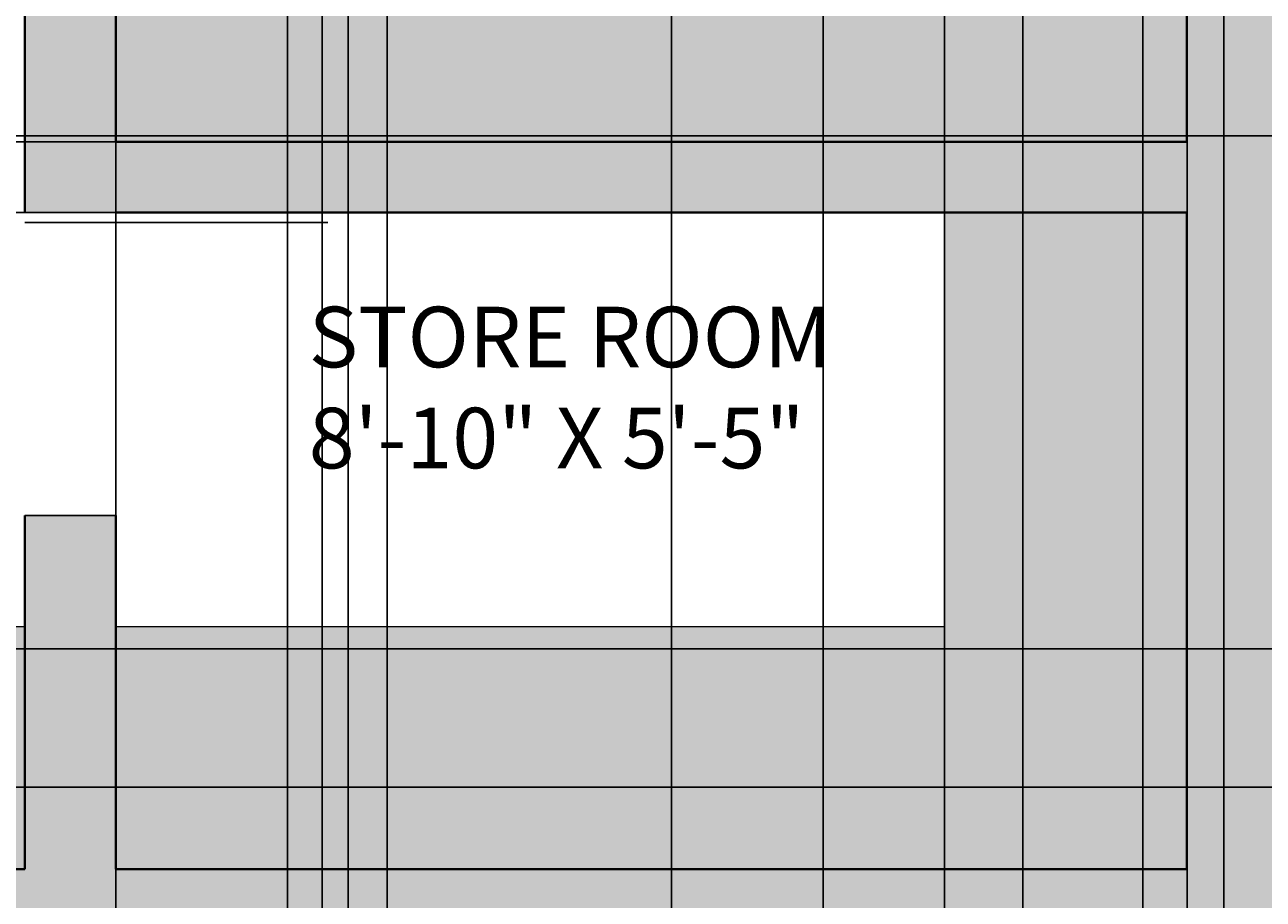
# Model space of a CAD drawing. Units: inches. Extents: x 818 to 1898, y 976 to 2364.
# Tile 88 of 96: x 1591 to 1713, y 1873 to 1960. Entities that reach past the tile are written whole.
import ezdxf

# ---------------------------------------------------------------- set-up
doc = ezdxf.new("R2010")
doc.units = ezdxf.units.IN
doc.header["$LTSCALE"] = 5
doc.header["$MEASUREMENT"] = 0
for name, color, linetype, lineweight in [('A-ANNO-DIMS', 2, 'Continuous', 18), ('A-AREA-IDEN', 7, 'Continuous', 18), ('A-DOOR', 3, 'Continuous', 25), ('A-FLOR-CASE', 8, 'Continuous', 18), ('A-FLOR-CASE-PATT', 33, 'Continuous', 9), ('A-FURN-PATT', 8, 'Continuous', 9), ('A-WALL', 7, 'Continuous', 40)]:
    doc.layers.add(name, color=color, linetype=linetype, lineweight=lineweight)
doc.layers.add('A-WALL-PATT', color=251, linetype='Continuous', lineweight=13, true_color=0x636466)
doc.styles.get("Standard").update_dxf_attribs({"font": 'arial.ttf'})
doc.dimstyles.get("Standard").update_dxf_attribs({"dimtxt": 0.18, "dimasz": 0.18, "dimexe": 0.18, "dimexo": 0.0625, "dimgap": 0.09, "dimtad": 0, "dimtih": 1, "dimtoh": 1, "dimdec": 4, "dimzin": 0, "dimdsep": 46, "dimtxsty": 'Standard', "dimcen": 0.09, "dimadec": 0, "dimazin": 0, "dimtfac": 1, "dimtdec": 4, "dimtofl": 0, "dimtmove": 0, "dimatfit": 3, "dimfxl": 1, "dimtolj": 1, "dimtzin": 0, "dimarcsym": 0})

# ---------------------------------------------------------------- blocks, each defined once
blk = doc.blocks.new('*D85')
at = {"layer": 'A-ANNO-DIMS', "color": 0, "lineweight": -2, "ltscale": 5, "transparency": 16777216}
for p, q in [((1258.79, 2053.08), (1897.92, 2053.08)), ((1897.74, 2052.9), (1897.74, 1876.76)), ((1897.74, 1700.26), (1897.74, 1876.4)), ((1258.79, 1700.08), (1897.92, 1700.08))]:
    blk.add_line(p, q, dxfattribs=at)
at = {"layer": 'A-ANNO-DIMS', "color": 0, "ltscale": 5, "transparency": 16777216}
for points in [[(1897.71, 2052.9), (1897.77, 2052.9), (1897.74, 2053.08)], [(1897.71, 1700.26), (1897.77, 1700.26), (1897.74, 1700.08)]]:
    blk.add_solid(points, dxfattribs=at)
at = {"layer": 'Defpoints', "color": 0, "ltscale": 5, "transparency": 16777216}
for p in [(1258.73, 2053.08), (1897.74, 2053.08), (1258.73, 1700.08)]:
    blk.add_point(p, dxfattribs=at)
at = {"layer": 'A-ANNO-DIMS', "color": 0, "ltscale": 5, "transparency": 16777216, "insert": (1897.74, 1876.58), "char_height": 0.18, "attachment_point": 5}
blk.add_mtext('\\A1;353', dxfattribs=at)
blk = doc.blocks.new('*D102')
at = {"layer": 'A-ANNO-DIMS', "color": 0, "lineweight": -2, "ltscale": 5, "transparency": 16777216}
for p, q in [((1565.48, 1071.12), (1565.48, 2363.87)), ((1565.66, 2363.69), (1595.63, 2363.69)), ((1626.39, 2363.69), (1596.42, 2363.69)), ((1626.57, 1071.12), (1626.57, 2363.87))]:
    blk.add_line(p, q, dxfattribs=at)
at = {"layer": 'A-ANNO-DIMS', "color": 0, "ltscale": 5, "transparency": 16777216}
for points in [[(1565.66, 2363.72), (1565.66, 2363.66), (1565.48, 2363.69)], [(1626.39, 2363.72), (1626.39, 2363.66), (1626.57, 2363.69)]]:
    blk.add_solid(points, dxfattribs=at)
at = {"layer": 'Defpoints', "color": 0, "ltscale": 5, "transparency": 16777216}
for p in [(1626.57, 2363.69), (1565.48, 1071.06), (1626.57, 1071.06)]:
    blk.add_point(p, dxfattribs=at)
at = {"layer": 'A-ANNO-DIMS', "color": 0, "ltscale": 5, "transparency": 16777216, "insert": (1596.03, 2363.69), "char_height": 0.18, "attachment_point": 5}
blk.add_mtext('\\A1;61.09', dxfattribs=at)
blk = doc.blocks.new('*D103')
at = {"layer": 'A-ANNO-DIMS', "color": 0, "lineweight": -2, "ltscale": 5, "transparency": 16777216}
for p, q in [((1626.57, 1071.12), (1626.57, 2363.87)), ((1626.75, 2363.69), (1657.7, 2363.69)), ((1689.29, 2363.69), (1658.35, 2363.69)), ((1689.47, 1071.12), (1689.47, 2363.87))]:
    blk.add_line(p, q, dxfattribs=at)
at = {"layer": 'A-ANNO-DIMS', "color": 0, "ltscale": 5, "transparency": 16777216}
for points in [[(1626.75, 2363.72), (1626.75, 2363.66), (1626.57, 2363.69)], [(1689.29, 2363.72), (1689.29, 2363.66), (1689.47, 2363.69)]]:
    blk.add_solid(points, dxfattribs=at)
at = {"layer": 'Defpoints', "color": 0, "ltscale": 5, "transparency": 16777216}
for p in [(1689.47, 2363.69), (1626.57, 1071.06), (1689.47, 1071.06)]:
    blk.add_point(p, dxfattribs=at)
at = {"layer": 'A-ANNO-DIMS', "color": 0, "ltscale": 5, "transparency": 16777216, "insert": (1658.02, 2363.69), "char_height": 0.18, "attachment_point": 5}
blk.add_mtext('\\A1;62.9', dxfattribs=at)
blk = doc.blocks.new('*D104')
at = {"layer": 'A-ANNO-DIMS', "color": 0, "lineweight": -2, "ltscale": 5, "transparency": 16777216}
for p, q in [((1689.47, 1071.12), (1689.47, 2363.87)), ((1689.65, 2363.69), (1717.4, 2363.69)), ((1745.9, 2363.69), (1718.15, 2363.69)), ((1746.08, 1071.12), (1746.08, 2363.87))]:
    blk.add_line(p, q, dxfattribs=at)
at = {"layer": 'A-ANNO-DIMS', "color": 0, "ltscale": 5, "transparency": 16777216}
for points in [[(1689.65, 2363.72), (1689.65, 2363.66), (1689.47, 2363.69)], [(1745.9, 2363.72), (1745.9, 2363.66), (1746.08, 2363.69)]]:
    blk.add_solid(points, dxfattribs=at)
at = {"layer": 'Defpoints', "color": 0, "ltscale": 5, "transparency": 16777216}
for p in [(1746.08, 2363.69), (1689.47, 1071.06), (1746.08, 1071.06)]:
    blk.add_point(p, dxfattribs=at)
at = {"layer": 'A-ANNO-DIMS', "color": 0, "ltscale": 5, "transparency": 16777216, "insert": (1717.78, 2363.69), "char_height": 0.18, "attachment_point": 5}
blk.add_mtext('\\A1;56.61', dxfattribs=at)
blk = doc.blocks.new('*D121')
at = {"layer": 'A-ANNO-DIMS', "color": 0, "lineweight": -2, "ltscale": 5, "transparency": 16777216}
for p, q in [((1766.29, 1884.2), (818.03, 1884.2)), ((818.21, 1884.02), (818.21, 1841.14)), ((818.21, 1797.9), (818.21, 1840.78)), ((1766.29, 1797.72), (818.03, 1797.72))]:
    blk.add_line(p, q, dxfattribs=at)
at = {"layer": 'A-ANNO-DIMS', "color": 0, "ltscale": 5, "transparency": 16777216}
for points in [[(818.18, 1884.02), (818.24, 1884.02), (818.21, 1884.2)], [(818.18, 1797.9), (818.24, 1797.9), (818.21, 1797.72)]]:
    blk.add_solid(points, dxfattribs=at)
at = {"layer": 'Defpoints', "color": 0, "ltscale": 5, "transparency": 16777216}
for p in [(818.21, 1884.2), (1766.35, 1884.2), (1766.35, 1797.72)]:
    blk.add_point(p, dxfattribs=at)
at = {"layer": 'A-ANNO-DIMS', "color": 0, "ltscale": 5, "transparency": 16777216, "insert": (818.21, 1840.96), "char_height": 0.18, "attachment_point": 5}
blk.add_mtext('\\A1;86.49', dxfattribs=at)
blk = doc.blocks.new('*D154')
at = {"layer": 'A-ANNO-DIMS', "color": 0, "lineweight": -2, "ltscale": 5, "transparency": 16777216}
for p, q in [((1701.37, 1290.14), (1701.37, 2363.87)), ((1701.55, 2363.69), (1705.22, 2363.69)), ((1709.19, 2363.69), (1705.52, 2363.69)), ((1709.37, 1298.14), (1709.37, 2363.87))]:
    blk.add_line(p, q, dxfattribs=at)
at = {"layer": 'A-ANNO-DIMS', "color": 0, "ltscale": 5, "transparency": 16777216}
for points in [[(1701.55, 2363.72), (1701.55, 2363.66), (1701.37, 2363.69)], [(1709.19, 2363.72), (1709.19, 2363.66), (1709.37, 2363.69)]]:
    blk.add_solid(points, dxfattribs=at)
at = {"layer": 'Defpoints', "color": 0, "ltscale": 5, "transparency": 16777216}
for p in [(1709.37, 2363.69), (1709.37, 1298.08), (1701.37, 1290.08)]:
    blk.add_point(p, dxfattribs=at)
at = {"layer": 'A-ANNO-DIMS', "color": 0, "ltscale": 5, "transparency": 16777216, "insert": (1705.37, 2363.69), "char_height": 0.18, "attachment_point": 5}
blk.add_mtext('\\A1;8', dxfattribs=at)
blk = doc.blocks.new('*D173')
at = {"layer": 'A-ANNO-DIMS', "color": 0, "lineweight": -2, "ltscale": 5, "transparency": 16777216}
for p, q in [((1622.73, 1463.14), (1622.73, 2363.87)), ((1622.91, 2363.69), (1638.51, 2363.69)), ((1654.55, 2363.69), (1638.94, 2363.69)), ((1654.73, 1463.14), (1654.73, 2363.87))]:
    blk.add_line(p, q, dxfattribs=at)
at = {"layer": 'A-ANNO-DIMS', "color": 0, "ltscale": 5, "transparency": 16777216}
for points in [[(1622.91, 2363.72), (1622.91, 2363.66), (1622.73, 2363.69)], [(1654.55, 2363.72), (1654.55, 2363.66), (1654.73, 2363.69)]]:
    blk.add_solid(points, dxfattribs=at)
at = {"layer": 'Defpoints', "color": 0, "ltscale": 5, "transparency": 16777216}
for p in [(1654.73, 2363.69), (1622.73, 1463.08), (1654.73, 1463.08)]:
    blk.add_point(p, dxfattribs=at)
at = {"layer": 'A-ANNO-DIMS', "color": 0, "ltscale": 5, "transparency": 16777216, "insert": (1638.73, 2363.69), "char_height": 0.18, "attachment_point": 5}
blk.add_mtext('\\A1;32', dxfattribs=at)
blk = doc.blocks.new('*D174')
at = {"layer": 'A-ANNO-DIMS', "color": 0, "lineweight": -2, "ltscale": 5, "transparency": 16777216}
for p, q in [((1616.73, 1416.75), (1616.73, 2363.87)), ((1616.91, 2363.69), (1619.58, 2363.69)), ((1622.55, 2363.69), (1619.87, 2363.69)), ((1622.73, 1416.75), (1622.73, 2363.87))]:
    blk.add_line(p, q, dxfattribs=at)
at = {"layer": 'A-ANNO-DIMS', "color": 0, "ltscale": 5, "transparency": 16777216}
for points in [[(1616.91, 2363.72), (1616.91, 2363.66), (1616.73, 2363.69)], [(1622.55, 2363.72), (1622.55, 2363.66), (1622.73, 2363.69)]]:
    blk.add_solid(points, dxfattribs=at)
at = {"layer": 'Defpoints', "color": 0, "ltscale": 5, "transparency": 16777216}
for p in [(1622.73, 2363.69), (1616.73, 1416.69), (1622.73, 1416.69)]:
    blk.add_point(p, dxfattribs=at)
at = {"layer": 'A-ANNO-DIMS', "color": 0, "ltscale": 5, "transparency": 16777216, "insert": (1619.73, 2363.69), "char_height": 0.18, "attachment_point": 5}
blk.add_mtext('\\A1;6', dxfattribs=at)
blk = doc.blocks.new('*D175')
at = {"layer": 'A-ANNO-DIMS', "color": 0, "lineweight": -2, "ltscale": 5, "transparency": 16777216}
for p, q in [((1559.73, 1647.64), (1559.73, 2363.87)), ((1559.91, 2363.69), (1614.45, 2363.69)), ((1669.55, 2363.69), (1615.01, 2363.69)), ((1669.73, 1647.64), (1669.73, 2363.87))]:
    blk.add_line(p, q, dxfattribs=at)
at = {"layer": 'A-ANNO-DIMS', "color": 0, "ltscale": 5, "transparency": 16777216}
for points in [[(1559.91, 2363.72), (1559.91, 2363.66), (1559.73, 2363.69)], [(1669.55, 2363.72), (1669.55, 2363.66), (1669.73, 2363.69)]]:
    blk.add_solid(points, dxfattribs=at)
at = {"layer": 'Defpoints', "color": 0, "ltscale": 5, "transparency": 16777216}
for p in [(1669.73, 2363.69), (1559.73, 1647.58), (1669.73, 1647.58)]:
    blk.add_point(p, dxfattribs=at)
at = {"layer": 'A-ANNO-DIMS', "color": 0, "ltscale": 5, "transparency": 16777216, "insert": (1614.73, 2363.69), "char_height": 0.18, "attachment_point": 5}
blk.add_mtext('\\A1;110', dxfattribs=at)
blk = doc.blocks.new('*D195')
at = {"layer": 'A-ANNO-DIMS', "color": 0, "lineweight": -2, "ltscale": 5, "transparency": 16777216}
for p, q in [((1681.73, 1379.14), (1681.73, 2363.87)), ((1681.91, 2363.69), (1693.51, 2363.69)), ((1705.55, 2363.69), (1693.95, 2363.69)), ((1705.73, 1355.14), (1705.73, 2363.87))]:
    blk.add_line(p, q, dxfattribs=at)
at = {"layer": 'A-ANNO-DIMS', "color": 0, "ltscale": 5, "transparency": 16777216}
for points in [[(1681.91, 2363.72), (1681.91, 2363.66), (1681.73, 2363.69)], [(1705.55, 2363.72), (1705.55, 2363.66), (1705.73, 2363.69)]]:
    blk.add_solid(points, dxfattribs=at)
at = {"layer": 'Defpoints', "color": 0, "ltscale": 5, "transparency": 16777216}
for p in [(1705.73, 2363.69), (1681.73, 1379.08), (1705.73, 1355.08)]:
    blk.add_point(p, dxfattribs=at)
at = {"layer": 'A-ANNO-DIMS', "color": 0, "ltscale": 5, "transparency": 16777216, "insert": (1693.73, 2363.69), "char_height": 0.18, "attachment_point": 5}
blk.add_mtext('\\A1;24', dxfattribs=at)
blk = doc.blocks.new('*D203')
at = {"layer": 'A-ANNO-DIMS', "color": 0, "lineweight": -2, "ltscale": 5, "transparency": 16777216}
for p, q in [((1599.73, 1876.14), (1599.73, 2363.87)), ((1599.91, 2363.69), (1652.44, 2363.69)), ((1705.55, 2363.69), (1653.01, 2363.69)), ((1705.73, 1876.14), (1705.73, 2363.87))]:
    blk.add_line(p, q, dxfattribs=at)
at = {"layer": 'A-ANNO-DIMS', "color": 0, "ltscale": 5, "transparency": 16777216}
for points in [[(1599.91, 2363.72), (1599.91, 2363.66), (1599.73, 2363.69)], [(1705.55, 2363.72), (1705.55, 2363.66), (1705.73, 2363.69)]]:
    blk.add_solid(points, dxfattribs=at)
at = {"layer": 'Defpoints', "color": 0, "ltscale": 5, "transparency": 16777216}
for p in [(1705.73, 2363.69), (1599.73, 1876.08), (1705.73, 1876.08)]:
    blk.add_point(p, dxfattribs=at)
at = {"layer": 'A-ANNO-DIMS', "color": 0, "ltscale": 5, "transparency": 16777216, "insert": (1652.73, 2363.69), "char_height": 0.18, "attachment_point": 5}
blk.add_mtext('\\A1;106', dxfattribs=at)
blk = doc.blocks.new('*D204')
at = {"layer": 'A-ANNO-DIMS', "color": 0, "lineweight": -2, "ltscale": 5, "transparency": 16777216}
for p, q in [((1714.79, 2053.08), (1897.92, 2053.08)), ((1897.74, 2052.9), (1897.74, 1960.26)), ((1897.74, 1867.26), (1897.74, 1959.9)), ((1705.79, 1867.08), (1897.92, 1867.08))]:
    blk.add_line(p, q, dxfattribs=at)
at = {"layer": 'A-ANNO-DIMS', "color": 0, "ltscale": 5, "transparency": 16777216}
for points in [[(1897.71, 2052.9), (1897.77, 2052.9), (1897.74, 2053.08)], [(1897.71, 1867.26), (1897.77, 1867.26), (1897.74, 1867.08)]]:
    blk.add_solid(points, dxfattribs=at)
at = {"layer": 'Defpoints', "color": 0, "ltscale": 5, "transparency": 16777216}
for p in [(1714.73, 2053.08), (1897.74, 2053.08), (1705.73, 1867.08)]:
    blk.add_point(p, dxfattribs=at)
at = {"layer": 'A-ANNO-DIMS', "color": 0, "ltscale": 5, "transparency": 16777216, "insert": (1897.74, 1960.08), "char_height": 0.18, "attachment_point": 5}
blk.add_mtext('\\A1;186', dxfattribs=at)
blk = doc.blocks.new('*D211')
at = {"layer": 'A-ANNO-DIMS', "color": 0, "lineweight": -2, "ltscale": 5, "transparency": 16777216}
for p, q in [((1599.66265, 1948.078237), (818.025912, 1948.078237)), ((818.205912, 1947.898237), (818.205912, 1944.758237)), ((818.205912, 1941.258237), (818.205912, 1944.398237)), ((1599.66265, 1941.078237), (818.025912, 1941.078237))]:
    blk.add_line(p, q, dxfattribs=at)
at = {"layer": 'A-ANNO-DIMS', "color": 0, "ltscale": 5, "transparency": 16777216}
for points in [[(818.175912, 1947.898237), (818.235912, 1947.898237), (818.205912, 1948.078237)], [(818.175912, 1941.258237), (818.235912, 1941.258237), (818.205912, 1941.078237)]]:
    blk.add_solid(points, dxfattribs=at)
at = {"layer": 'Defpoints', "color": 0, "ltscale": 5, "transparency": 16777216}
for p in [(818.205912, 1948.078237), (1599.72515, 1948.078237), (1599.72515, 1941.078237)]:
    blk.add_point(p, dxfattribs=at)
at = {"layer": 'A-ANNO-DIMS', "color": 0, "ltscale": 5, "transparency": 16777216, "insert": (818.205912, 1944.578237), "char_height": 0.18, "attachment_point": 5}
blk.add_mtext('\\A1;7', dxfattribs=at)
blk = doc.blocks.new('*D212')
at = {"layer": 'A-ANNO-DIMS', "color": 0, "lineweight": -2, "ltscale": 5, "transparency": 16777216}
for p, q in [((1681.73, 1900.02), (1681.73, 975.66)), ((1705.73, 1876.02), (1705.73, 975.66)), ((1681.91, 975.84), (1693.51, 975.84)), ((1705.55, 975.84), (1693.95, 975.84))]:
    blk.add_line(p, q, dxfattribs=at)
at = {"layer": 'A-ANNO-DIMS', "color": 0, "ltscale": 5, "transparency": 16777216}
for points in [[(1681.91, 975.87), (1681.91, 975.81), (1681.73, 975.84)], [(1705.55, 975.87), (1705.55, 975.81), (1705.73, 975.84)]]:
    blk.add_solid(points, dxfattribs=at)
at = {"layer": 'Defpoints', "color": 0, "ltscale": 5, "transparency": 16777216}
for p in [(1681.73, 1900.08), (1705.73, 1876.08), (1705.73, 975.84)]:
    blk.add_point(p, dxfattribs=at)
at = {"layer": 'A-ANNO-DIMS', "color": 0, "ltscale": 5, "transparency": 16777216, "insert": (1693.73, 975.84), "char_height": 0.18, "attachment_point": 5}
blk.add_mtext('\\A1;24', dxfattribs=at)
blk = doc.blocks.new('*D229')
at = {"layer": 'A-ANNO-DIMS', "color": 0, "lineweight": -2, "ltscale": 5, "transparency": 16777216}
for p, q in [((1599.73, 2044.02), (1599.73, 975.66)), ((1620.14, 2036.06), (1620.14, 975.66)), ((1599.91, 975.84), (1609.47, 975.84)), ((1619.96, 975.84), (1610.4, 975.84))]:
    blk.add_line(p, q, dxfattribs=at)
at = {"layer": 'A-ANNO-DIMS', "color": 0, "ltscale": 5, "transparency": 16777216}
for points in [[(1599.91, 975.87), (1599.91, 975.81), (1599.73, 975.84)], [(1619.96, 975.87), (1619.96, 975.81), (1620.14, 975.84)]]:
    blk.add_solid(points, dxfattribs=at)
at = {"layer": 'Defpoints', "color": 0, "ltscale": 5, "transparency": 16777216}
for p in [(1599.73, 2044.08), (1620.14, 2036.12), (1620.14, 975.84)]:
    blk.add_point(p, dxfattribs=at)
at = {"layer": 'A-ANNO-DIMS', "color": 0, "ltscale": 5, "transparency": 16777216, "insert": (1609.93, 975.84), "char_height": 0.18, "attachment_point": 5}
blk.add_mtext('\\A1;20.416', dxfattribs=at)
blk = doc.blocks.new('*D239')
at = {"layer": 'A-ANNO-DIMS', "color": 0, "lineweight": -2, "ltscale": 5, "transparency": 16777216}
for p, q in [((1483.61, 1979.24), (1897.92, 1979.24)), ((1897.74, 1979.06), (1897.74, 1964.13)), ((1897.74, 1948.84), (1897.74, 1963.77)), ((1483.61, 1948.66), (1897.92, 1948.66))]:
    blk.add_line(p, q, dxfattribs=at)
at = {"layer": 'A-ANNO-DIMS', "color": 0, "ltscale": 5, "transparency": 16777216}
for points in [[(1897.71, 1979.06), (1897.77, 1979.06), (1897.74, 1979.24)], [(1897.71, 1948.84), (1897.77, 1948.84), (1897.74, 1948.66)]]:
    blk.add_solid(points, dxfattribs=at)
at = {"layer": 'Defpoints', "color": 0, "ltscale": 5, "transparency": 16777216}
for p in [(1483.55, 1979.24), (1897.74, 1979.24), (1483.55, 1948.66)]:
    blk.add_point(p, dxfattribs=at)
at = {"layer": 'A-ANNO-DIMS', "color": 0, "ltscale": 5, "transparency": 16777216, "insert": (1897.74, 1963.95), "char_height": 0.18, "attachment_point": 5}
blk.add_mtext('\\A1;30.584', dxfattribs=at)
blk = doc.blocks.new('*D275')
at = {"layer": 'A-ANNO-DIMS', "color": 0, "lineweight": -2, "ltscale": 5, "transparency": 16777216}
for p, q in [((1377.84, 1897.87), (1897.92, 1897.87)), ((1897.74, 1897.69), (1897.74, 1875.99)), ((1897.74, 1853.93), (1897.74, 1875.63)), ((1377.84, 1853.75), (1897.92, 1853.75))]:
    blk.add_line(p, q, dxfattribs=at)
at = {"layer": 'A-ANNO-DIMS', "color": 0, "ltscale": 5, "transparency": 16777216}
for points in [[(1897.71, 1897.69), (1897.77, 1897.69), (1897.74, 1897.87)], [(1897.71, 1853.93), (1897.77, 1853.93), (1897.74, 1853.75)]]:
    blk.add_solid(points, dxfattribs=at)
at = {"layer": 'Defpoints', "color": 0, "ltscale": 5, "transparency": 16777216}
for p in [(1377.78, 1897.87), (1897.74, 1897.87), (1377.78, 1853.75)]:
    blk.add_point(p, dxfattribs=at)
at = {"layer": 'A-ANNO-DIMS', "color": 0, "ltscale": 5, "transparency": 16777216, "insert": (1897.74, 1875.81), "char_height": 0.18, "attachment_point": 5}
blk.add_mtext('\\A1;44.12', dxfattribs=at)
blk = doc.blocks.new('*D282')
at = {"layer": 'A-ANNO-DIMS', "color": 0, "lineweight": -2, "ltscale": 5, "transparency": 16777216}
for p, q in [((1422.08, 2081.19), (1897.92, 2081.19)), ((1897.74, 2081.01), (1897.74, 1884.32)), ((1897.74, 1687.26), (1897.74, 1883.95)), ((1463.79, 1687.08), (1897.92, 1687.08))]:
    blk.add_line(p, q, dxfattribs=at)
at = {"layer": 'A-ANNO-DIMS', "color": 0, "ltscale": 5, "transparency": 16777216}
for points in [[(1897.71, 2081.01), (1897.77, 2081.01), (1897.74, 2081.19)], [(1897.71, 1687.26), (1897.77, 1687.26), (1897.74, 1687.08)]]:
    blk.add_solid(points, dxfattribs=at)
at = {"layer": 'Defpoints', "color": 0, "ltscale": 5, "transparency": 16777216}
for p in [(1422.02, 2081.19), (1897.74, 2081.19), (1463.73, 1687.08)]:
    blk.add_point(p, dxfattribs=at)
at = {"layer": 'A-ANNO-DIMS', "color": 0, "ltscale": 5, "transparency": 16777216, "insert": (1897.74, 1884.13), "char_height": 0.18, "attachment_point": 5}
blk.add_mtext('\\A1;394.1', dxfattribs=at)

msp = doc.modelspace()

# ---------------------------------------------------------------- hatches: boundary and pattern name
at = {"layer": 'A-FLOR-CASE-PATT', "ltscale": 5}
h = msp.add_hatch(color=256, dxfattribs=at)
h.dxf.hatch_style = 1
h.paths.add_polyline_path([(1705.7251, 1941.0782), (1681.7251, 1941.0782), (1681.7251, 1900.0782), (1599.7251, 1900.0782), (1599.7251, 1876.0782), (1705.7251, 1876.0782)])
h.paths.add_polyline_path([(1457.7252, 1409.1177), (1457.7252, 1526.6712), (1439.7252, 1526.6712), (1439.7252, 1457.5313), (1446.3307, 1457.5313), (1446.3307, 1468.9514), (1446.8307, 1470.665), (1446.8307, 1469.665), (1446.8307, 1468.9514), (1446.8307, 1456.8361), (1446.8307, 1444.7258), (1446.8307, 1443.3338), (1446.3307, 1444.7258), (1446.3307, 1456.8361), (1439.7252, 1456.8361), (1439.7252, 1355.0782), (1463.7251, 1355.0782), (1463.7251, 1367.3287), (1458.0475, 1367.3287, -0.23606798), (1457.0475, 1369.3287), (1456.0475, 1369.3287, -0.11764706), (1456.0475, 1386.3287), (1457.0475, 1386.3287, -0.23606798), (1458.0475, 1388.3287), (1463.7251, 1388.3287), (1463.7251, 1389.3211)])
h.paths.add_polyline_path([(1341.2593, 1534.0782), (1246.9377, 1534.0782), (1246.9377, 1510.0782), (1341.2593, 1510.0782)])
h.paths.add_polyline_path([(1288.8272, 1519.927), (1289.8272, 1519.927), (1290.5408, 1519.927), (1302.6561, 1519.927), (1314.7664, 1519.927), (1316.1584, 1519.927), (1314.7664, 1519.427), (1302.6561, 1519.427), (1302.6561, 1512.8214), (1301.9609, 1512.8214), (1301.9609, 1519.427), (1290.5408, 1519.427)], flags=16)
h.paths.add_polyline_path([(1377.7791, 1867.0782), (1344.5531, 1867.0782), (1344.5531, 1860.4726), (1355.9731, 1860.4726), (1357.6867, 1859.9726), (1356.6867, 1859.9726), (1355.9731, 1859.9726), (1343.8579, 1859.9726), (1331.7475, 1859.9726), (1330.3556, 1859.9726), (1331.7475, 1860.4726), (1343.8579, 1860.4726), (1343.8579, 1867.0782), (1311.3271, 1867.0782), (1311.3271, 1853.7496), (1377.7791, 1853.7496)])
h.paths.add_polyline_path([(1301.148, 1610.7299, -0.46196039), (1314.4882, 1599.3725, -0.19222541), (1311.3254, 1591.4497, 0.54791519), (1336.8832, 1607.7707, 0.92061359)])
h.paths.add_polyline_path([(1370.719, 1780.5695, 1), (1332.478, 1780.5695, 1)])
h.paths.add_polyline_path([(1705.7251, 1463.0782), (1681.7251, 1463.0782), (1681.7251, 1379.0782), (1622.7251, 1379.0782), (1622.7251, 1355.0782), (1705.7251, 1355.0782)])
h.paths.add_polyline_path([(1658.1052, 1359.2188), (1658.1786, 1359.2188), (1658.1786, 1373.8763), (1658.1052, 1373.9202)], flags=16)
h.paths.add_polyline_path([(1686.9271, 1409.9311), (1686.8832, 1409.8578), (1701.5845, 1409.8578), (1701.5845, 1409.9311)], flags=16)
h.paths.add_polyline_path([(1637.1266, 1359.2188), (1637.2, 1359.2188), (1637.2, 1373.8763), (1637.1266, 1373.9202)], flags=16)
at = {"layer": 'A-FURN-PATT', "ltscale": 5}
h = msp.add_hatch(color=256, dxfattribs=at)
h.dxf.hatch_style = 1
h.paths.add_polyline_path([(1341.9997, 1981.5338), (1317.9034, 2001.8247), (1314.2595, 2001.8247), (1314.2595, 2004.893), (1310.1046, 2008.3917), (1303.9314, 2008.3917), (1303.9314, 1953.0408), (1308.1629, 1953.0408), (1314.2595, 1958.1746), (1314.2595, 1959.6079), (1315.9616, 1959.6079)])
h.paths.add_polyline_path([(1341.9997, 1981.5338), (1315.9616, 1959.6079), (1336.7936, 1959.6079), (1336.7936, 1953.0408), (1345.3966, 1953.0408), (1345.3966, 1959.6079), (1368.0379, 1959.6079)])
h.paths.add_polyline_path([(1402.518, 2008.3917), (1398.8475, 2008.3917), (1398.8475, 2001.8247), (1376.3134, 2001.8247), (1376.3134, 2008.3917), (1373.8948, 2008.3917), (1367.9307, 2003.3695), (1367.9307, 2001.8247), (1366.0961, 2001.8247), (1341.9997, 1981.5338), (1368.0379, 1959.6079), (1375.8366, 1953.0408), (1376.3134, 1953.0408), (1376.3134, 1959.6079), (1398.8475, 1959.6079), (1398.8475, 1953.0408), (1402.518, 1953.0408)])
h.paths.add_polyline_path([(1366.0961, 2001.8247), (1345.3966, 2001.8247), (1345.3966, 2008.3917), (1336.7936, 2008.3917), (1336.7936, 2001.8247), (1317.9034, 2001.8247), (1341.9997, 1981.5338)])
h.paths.add_polyline_path([(1336.7936, 1959.6079), (1315.9616, 1959.6079), (1314.2595, 1958.1746), (1314.2595, 1953.0408), (1336.7936, 1953.0408)], flags=17)
h.paths.add_polyline_path([(1367.9307, 1959.6079), (1345.3966, 1959.6079), (1345.3966, 1953.0408), (1367.9307, 1953.0408)], flags=17)
h.paths.add_polyline_path([(1398.8475, 1959.6079), (1376.3134, 1959.6079), (1376.3134, 1953.0408), (1398.8475, 1953.0408)], flags=17)
h.paths.add_polyline_path([(1368.0379, 1959.6079), (1367.9307, 1959.6079), (1367.9307, 1953.0408), (1375.8366, 1953.0408)], flags=17)
h.paths.add_polyline_path([(1314.2595, 1958.1746), (1308.1629, 1953.0408), (1314.2595, 1953.0408)], flags=17)
h.paths.add_polyline_path([(1315.9616, 1959.6079), (1314.2595, 1959.6079), (1314.2595, 1958.1746)], flags=16)
h.paths.add_polyline_path([(1314.2595, 2008.3917), (1310.1046, 2008.3917), (1314.2595, 2004.893)], flags=17)
h.paths.add_polyline_path([(1336.7936, 2008.3917), (1314.2595, 2008.3917), (1314.2595, 2004.893), (1317.9034, 2001.8247), (1336.7936, 2001.8247)], flags=17)
h.paths.add_polyline_path([(1314.2595, 2004.893), (1314.2595, 2001.8247), (1317.9034, 2001.8247)], flags=16)
h.paths.add_polyline_path([(1367.9307, 2008.3917), (1345.3966, 2008.3917), (1345.3966, 2001.8247), (1366.0961, 2001.8247), (1367.9307, 2003.3695)], flags=17)
h.paths.add_polyline_path([(1398.8475, 2008.3917), (1376.3134, 2008.3917), (1376.3134, 2001.8247), (1398.8475, 2001.8247)], flags=17)
h.paths.add_polyline_path([(1373.8948, 2008.3917), (1367.9307, 2008.3917), (1367.9307, 2003.3695)], flags=17)
h.paths.add_polyline_path([(1367.9307, 2003.3695), (1366.0961, 2001.8247), (1367.9307, 2001.8247)], flags=16)
h.paths.add_polyline_path([(1546.1595, 2044.0782), (1451.7698, 2044.0782), (1451.7698, 2020.0782), (1546.1595, 2020.0782)])
h.paths.add_polyline_path([(1492.0729, 2040.001, 0.431429), (1491.8238, 2040.251), (1491.3087, 2040.251, 0.41521699), (1491.0729, 2040.001)], flags=16)
h.paths.add_polyline_path([(1481.8346, 2039.6036), (1511.886, 2039.6036), (1511.886, 2024.9917), (1481.8346, 2024.9917)], flags=16)
h.paths.add_polyline_path([(1491.0729, 2039.4857), (1491.0729, 2039.501), (1492.0729, 2039.501, -0.41174844), (1491.8401, 2039.251), (1491.8229, 2039.251), (1491.8229, 2039.2509, 0.43259178), (1492.0729, 2039.501), (1491.0729, 2039.501, 0.43260402), (1491.3229, 2039.2509), (1491.3229, 2039.251), (1491.325, 2039.251, -0.41658228)], flags=0)
h.paths.add_polyline_path([(1485.3701, 2030.9622), (1485.3701, 2034.3556, -0.41421356), (1488.3701, 2037.3556), (1490.3421, 2037.3556, -0.07791932), (1491.0729, 2038.751), (1495.0729, 2038.751, -0.31486788), (1496.07, 2037.1201, -0.30166092), (1497.9049, 2034.3556), (1497.9049, 2030.9622, -0.41421356), (1494.9049, 2027.9622), (1488.3701, 2027.9622, -0.41421356)], flags=0)
h.paths.add_polyline_path([(1490.3229, 2035.751, 0.26556482), (1491.3229, 2036.751), (1491.3229, 2037.126), (1491.0729, 2037.126, -0.79141832), (1490.5434, 2037.251, -0.79141832), (1491.0729, 2037.376), (1491.3229, 2037.376), (1491.3229, 2037.751), (1492.0729, 2037.751), (1492.0729, 2037.376), (1492.3229, 2037.376, -0.79141832), (1492.8524, 2037.251, -0.79141832), (1492.3229, 2037.126), (1492.1491, 2037.126, -0.08662632), (1492.5376, 2036.0294, 0.10704809), (1493.0729, 2035.751), (1490.3229, 2035.751)], flags=0)
h.paths.add_polyline_path([(1491.9774, 2037.251, -1), (1491.4184, 2037.251, -1)], flags=0)
h.paths.add_polyline_path([(1500.0743, 2028.6045), (1500.0743, 2029.4074), (1510.8414, 2029.4074), (1510.8414, 2028.6045)], flags=0)
h.paths.add_polyline_path([(1500.0743, 2030.5314), (1500.0743, 2031.3342), (1510.8414, 2031.3342), (1510.8414, 2030.5314)], flags=0)
h.paths.add_polyline_path([(1500.0743, 2032.94), (1500.0743, 2033.7428), (1510.8414, 2033.7428), (1510.8414, 2032.94)], flags=0)
h.paths.add_polyline_path([(1500.0743, 2035.7499), (1500.0743, 2036.5528), (1510.8414, 2036.5528), (1510.8414, 2035.7499)], flags=0)
h.paths.add_polyline_path([(1590.7252, 2044.0782), (1576.1595, 2044.0782), (1576.1595, 2020.0782), (1590.7252, 2020.0782)])
h.paths.add_polyline_path([(1668.4429, 2044.0782), (1599.7251, 2044.0782), (1599.7251, 2020.0782), (1668.4429, 2020.0782)])
h.paths.add_polyline_path([(1621.2588, 2040.001, 0.431429), (1621.0097, 2040.251), (1620.4946, 2040.251, 0.41521699), (1620.2588, 2040.001)], flags=16)
h.paths.add_polyline_path([(1611.0205, 2024.9917), (1611.0205, 2039.6036), (1641.0719, 2039.6036), (1641.0719, 2024.9917)], flags=16)
h.paths.add_polyline_path([(1620.2588, 2039.4857), (1620.2588, 2039.501), (1621.2588, 2039.501, -0.41174844), (1621.026, 2039.251), (1621.0088, 2039.251), (1621.0088, 2039.2509, 0.43259178), (1621.2588, 2039.501), (1620.2588, 2039.501, 0.43260402), (1620.5088, 2039.2509), (1620.5088, 2039.251), (1620.5109, 2039.251, -0.41658228)], flags=0)
h.paths.add_polyline_path([(1614.556, 2030.9622), (1614.556, 2034.3556, -0.41421356), (1617.556, 2037.3556), (1619.528, 2037.3556, -0.07791932), (1620.2588, 2038.751), (1624.2588, 2038.751, -0.31486788), (1625.2559, 2037.1201, -0.30166092), (1627.0908, 2034.3556), (1627.0908, 2030.9622, -0.41421356), (1624.0908, 2027.9622), (1617.556, 2027.9622, -0.41421356)], flags=0)
h.paths.add_polyline_path([(1619.5088, 2035.751, 0.26556482), (1620.5088, 2036.751), (1620.5088, 2037.126), (1620.2588, 2037.126, -0.79141832), (1619.7293, 2037.251, -0.79141832), (1620.2588, 2037.376), (1620.5088, 2037.376), (1620.5088, 2037.751), (1621.2588, 2037.751), (1621.2588, 2037.376), (1621.5088, 2037.376, -0.79141832), (1622.0383, 2037.251, -0.79141832), (1621.5088, 2037.126), (1621.335, 2037.126, -0.08662632), (1621.7235, 2036.0294, 0.10704809), (1622.2588, 2035.751), (1619.5088, 2035.751)], flags=0)
h.paths.add_polyline_path([(1620.6043, 2037.251, -1), (1621.1633, 2037.251, -1)], flags=0)
h.paths.add_polyline_path([(1629.2602, 2028.6045), (1629.2602, 2029.4074), (1640.0273, 2029.4074), (1640.0273, 2028.6045)], flags=0)
h.paths.add_polyline_path([(1629.2602, 2030.5314), (1629.2602, 2031.3342), (1640.0273, 2031.3342), (1640.0273, 2030.5314)], flags=0)
h.paths.add_polyline_path([(1629.2602, 2032.94), (1629.2602, 2033.7428), (1640.0273, 2033.7428), (1640.0273, 2032.94)], flags=0)
h.paths.add_polyline_path([(1629.2602, 2035.7499), (1629.2602, 2036.5528), (1640.0273, 2036.5528), (1640.0273, 2035.7499)], flags=0)
h.paths.add_polyline_path([(1705.7251, 2044.0782), (1698.4429, 2044.0782), (1698.4429, 2020.0782), (1705.7251, 2020.0782)])
h.paths.add_polyline_path([(1705.7251, 1972.0782), (1599.7251, 1972.0782), (1599.7251, 1948.0782), (1705.7251, 1948.0782)])
h.paths.add_polyline_path([(1550.0109, 1979.2444), (1483.5451, 1979.2444), (1483.5451, 1948.6602), (1550.0109, 1948.6602)])
h.paths.add_polyline_path([(1490.2586, 1948.6602), (1488.2586, 1948.6602), (1488.2586, 1941.1742, 0.41421356), (1491.2586, 1938.1742), (1500.7446, 1938.1742, -0.41421356)])
h.paths.add_polyline_path([(1513.2306, 1941.1742), (1513.2306, 1948.6602), (1511.2306, 1948.6602, -0.41421356), (1500.7446, 1938.1742), (1510.2306, 1938.1742, 0.41421356)])
h.paths.add_polyline_path([(1518.778, 1948.6602), (1516.778, 1948.6602), (1516.778, 1941.1742, 0.41421356), (1519.778, 1938.1742), (1529.264, 1938.1742, -0.41421356)])
h.paths.add_polyline_path([(1541.75, 1941.1742), (1541.75, 1948.6602), (1539.75, 1948.6602, -0.41421356), (1529.264, 1938.1742), (1538.75, 1938.1742, 0.41421356)])
h.paths.add_polyline_path([(1590.7252, 1900.0782), (1519.6413, 1900.0782), (1519.6413, 1876.0782), (1590.7252, 1876.0782)])
at = {"layer": 'A-WALL-PATT', "ltscale": 5}
h = msp.add_hatch(color=256, dxfattribs=at)
h.dxf.hatch_style = 1
h.paths.add_polyline_path([(1267.7252, 1928.9218), (1258.7251, 1928.9218), (1258.7251, 1913.6401), (1250.3029, 1913.6401), (1250.3029, 1878.3919), (1258.7251, 1878.3919), (1258.7251, 1862.9652), (1267.7252, 1862.9652)])
h.paths.add_polyline_path([(1267.7252, 1814.9652), (1258.7251, 1814.9652), (1258.7251, 1755.3321), (1267.7252, 1755.3321)])
h.paths.add_polyline_path([(1463.7251, 1696.0782), (1267.7252, 1696.0782), (1267.7252, 1707.3321), (1258.7251, 1707.3321), (1258.7251, 1700.0782), (1251.9333, 1700.0782), (1251.9333, 1687.0782), (1463.7251, 1687.0782)])
h.paths.add_polyline_path([(1714.7251, 1717.3178), (1705.7251, 1717.3178), (1705.7251, 1696.0782), (1599.7251, 1696.0782), (1599.7251, 1790.0782), (1705.7251, 1790.0782), (1705.7251, 1785.6125), (1714.7251, 1785.6125), (1714.7251, 1827.2125), (1705.7251, 1827.2125), (1705.7251, 1802.0782), (1599.7251, 1802.0782), (1599.7251, 1867.0782), (1705.7251, 1867.0782), (1705.7251, 1857.2125), (1714.7251, 1857.2125), (1714.7251, 1930.0316), (1741.8409, 1930.0316), (1741.8409, 1935.0316), (1714.7251, 1935.0316), (1714.7251, 1957.0338), (1741.8409, 1957.0338), (1741.8409, 1962.0338), (1714.7251, 1962.0338), (1705.7251, 1962.0338), (1705.7251, 1948.0782), (1599.7251, 1948.0782), (1599.7251, 1981.0782), (1590.7252, 1981.0782), (1590.7252, 1941.0782), (1620.7252, 1941.0782), (1705.7251, 1941.0782), (1705.7251, 1876.0782), (1599.7251, 1876.0782), (1599.7251, 1911.0782), (1590.7252, 1911.0782), (1590.7252, 1876.0782), (1429.2252, 1876.0782), (1429.2252, 1867.0782), (1511.7252, 1867.0782), (1528.593, 1867.0782), (1595.7252, 1867.0782), (1595.7252, 1773.0782), (1520.7252, 1773.0782), (1520.7252, 1837.5823), (1532.593, 1837.5823), (1532.593, 1867.0782), (1528.593, 1867.0782), (1528.593, 1841.5823), (1511.7252, 1841.5823), (1511.7252, 1744.9714), (1520.7252, 1744.9714), (1520.7252, 1761.0782), (1595.7252, 1761.0782), (1595.7252, 1696.0782), (1520.7252, 1696.0782), (1520.7252, 1716.0454), (1511.7252, 1716.0454), (1511.7252, 1696.0782), (1511.7252, 1687.0782), (1714.7251, 1687.0782)])
h.paths.add_polyline_path([(1714.7251, 2053.0782), (1714.7251, 2081.1881), (1709.7252, 2081.1881), (1709.7252, 2053.0782), (1681.6446, 2053.0782), (1681.6446, 2081.1881), (1676.6446, 2081.1881), (1676.6446, 2053.0782), (1538.5155, 2053.0782), (1538.5155, 2044.0782), (1590.7252, 2044.0782), (1590.7252, 2011.0782), (1599.7251, 2011.0782), (1599.7251, 2044.0782), (1705.7251, 2044.0782), (1705.7251, 2014.5114), (1714.7251, 2014.5114)])
h.paths.add_polyline_path([(1485.1216, 2053.0782), (1422.02, 2053.0782), (1422.02, 2081.1881), (1413.02, 2081.1881), (1413.02, 2053.0782), (1399.6356, 2053.0782), (1399.6356, 2081.1881), (1390.6356, 2081.1881), (1390.6356, 2053.0782), (1388.0315, 2053.0782), (1388.0315, 2044.0782), (1416.2743, 2044.0782), (1485.1216, 2044.0782)])
h.paths.add_polyline_path([(1330.305, 2053.0782), (1258.7251, 2053.0782), (1258.7251, 2019.2871), (1267.7252, 2019.2871), (1267.7252, 2044.0782), (1330.305, 2044.0782)])
h.paths.add_polyline_path([(1258.7251, 2053.0782), (1214.6577, 2053.0782), (1214.6577, 2044.0782), (1258.7251, 2044.0782)])
h.paths.add_polyline_path([(1214.6577, 2053.0782), (1180.349, 2053.0782), (1180.349, 2044.0782), (1214.6577, 2044.0782)])
h.paths.add_polyline_path([(1714.7251, 1639.5782), (1741.8409, 1639.5782), (1741.8409, 1643.5782), (1714.7251, 1643.5782), (1714.7251, 1649.9029), (1705.7251, 1649.9029), (1705.7251, 1600.0782), (1477.7252, 1600.0782), (1477.7252, 1591.0782), (1520.7252, 1591.0782), (1616.7251, 1591.0782), (1616.7251, 1416.6857), (1622.7251, 1416.6857), (1622.7251, 1463.0782), (1624.7252, 1463.0782), (1624.7252, 1467.0782), (1622.7251, 1467.0782), (1622.7251, 1591.0782), (1705.7251, 1591.0782), (1705.7251, 1545.0782), (1714.7251, 1545.0782), (1741.8409, 1545.0782), (1741.8409, 1549.0782), (1714.7251, 1549.0782), (1714.7251, 1593.9175), (1737.8409, 1593.9175), (1737.8409, 1597.9175), (1714.7251, 1597.9175)])
h.paths.add_polyline_path([(1674.9024, 2060.7419), (1714.7045, 2060.7419), (1714.7045, 2073.1061), (1674.9024, 2073.1061)], flags=25)
h.paths.add_polyline_path([(1394.5468, 2061.6618), (1422.2344, 2061.6618), (1422.2344, 2074.0261), (1394.5468, 2074.0261)], flags=24)

# ---------------------------------------------------------------- linework, layer by layer
at = {"layer": 'A-DOOR'}
for p, q in [((1599.7251, 1941.0782), (1590.7252, 1941.0782)), ((1590.7252, 1941.0782), (1620.7252, 1941.0782)), ((1590.7252, 1940.0782), (1620.7252, 1940.0782)), ((1599.7251, 1911.0782), (1590.7252, 1911.0782))]:
    msp.add_line(p, q, dxfattribs=at)
at = {"layer": 'A-FLOR-CASE'}
for p, q in [((1681.7251, 1941.0782), (1681.7251, 1900.0782)), ((1519.6413, 1900.0782), (1590.7252, 1900.0782)), ((1599.7251, 1900.0782), (1681.7251, 1900.0782))]:
    msp.add_line(p, q, dxfattribs=at)
at = {"layer": 'A-WALL'}
for p, q in [((1705.7251, 2044.0782), (1705.7251, 1948.0782)), ((1590.7252, 1981.0782), (1590.7252, 1941.0782)), ((1599.7251, 1981.0782), (1599.7251, 1948.0782)), ((1599.7251, 1981.0782), (1599.7251, 1948.0782)), ((1599.7251, 1948.0782), (1705.7251, 1948.0782)), ((1599.7251, 1941.0782), (1705.7251, 1941.0782)), ((1705.7251, 1941.0782), (1705.7251, 1876.0782)), ((1590.7252, 1911.0782), (1590.7252, 1876.0782)), ((1599.7251, 1911.0782), (1599.7251, 1876.0782)), ((1599.7251, 1911.0782), (1599.7251, 1876.0782)), ((1429.2252, 1876.0782), (1590.7252, 1876.0782)), ((1599.7251, 1876.0782), (1705.7251, 1876.0782))]:
    msp.add_line(p, q, dxfattribs=at)

# ---------------------------------------------------------------- texts
at = {"layer": 'A-AREA-IDEN', "ltscale": 5, "insert": (1618.8278, 1931.7478), "char_height": 6, "attachment_point": 1}
msp.add_mtext_dynamic_manual_height_columns('STORE ROOM\\P8\'-10" X 5\'-5"', width=118.992422, gutter_width=1, heights=[0], dxfattribs=at)

# ---------------------------------------------------------------- dimensions: what is measured, and where the dimension line sits
at = {"layer": 'A-ANNO-DIMS', "ltscale": 5}
for base, p1, p2, override, picture, middle in [((1669.7251, 2363.6929), (1559.7251, 1647.5782), (1669.7251, 1647.5782), {"dimdec": 0, "dimlfac": 1, "dimrnd": 0, "dimzin": 0, "dimdsep": 46, "dimlunit": 2}, '*D175', (1614.7251, 2363.6929)), ((1626.5748, 2363.6929), (1565.4835, 1071.0552), (1626.5748, 1071.0552), {"dimdec": 2, "dimlfac": 1, "dimrnd": 0, "dimzin": 0, "dimdsep": 46, "dimlunit": 2}, '*D102', (1596.0291, 2363.6929)), ((1705.7251, 2363.6929), (1599.7251, 1876.0782), (1705.7251, 1876.0782), {"dimdec": 0, "dimlfac": 1, "dimrnd": 0, "dimzin": 0, "dimdsep": 46, "dimlunit": 2}, '*D203', (1652.7251, 2363.6929)), ((1622.7251, 2363.6929), (1616.7251, 1416.6857), (1622.7251, 1416.6857), {"dimdec": 0, "dimlfac": 1, "dimrnd": 0, "dimzin": 0, "dimdsep": 46, "dimlunit": 2}, '*D174', (1619.7251, 2363.6929)), ((1654.7251, 2363.6929), (1622.7251, 1463.0782), (1654.7251, 1463.0782), {"dimdec": 0, "dimlfac": 1, "dimrnd": 0, "dimzin": 0, "dimdsep": 46, "dimlunit": 2}, '*D173', (1638.7251, 2363.6929)), ((1689.4714, 2363.6929), (1626.5748, 1071.0552), (1689.4714, 1071.0552), {"dimdec": 1, "dimlfac": 1, "dimrnd": 0, "dimzin": 0, "dimdsep": 46, "dimlunit": 2}, '*D103', (1658.0231, 2363.6929)), ((1705.7251, 2363.6929), (1681.7251, 1379.0782), (1705.7251, 1355.0782), {"dimdec": 0, "dimlfac": 1, "dimrnd": 0, "dimzin": 0, "dimdsep": 46, "dimlunit": 2}, '*D195', (1693.7251, 2363.6929)), ((1746.0831, 2363.6929), (1689.4714, 1071.0552), (1746.0831, 1071.0552), {"dimdec": 2, "dimlfac": 1, "dimrnd": 0, "dimzin": 0, "dimdsep": 46, "dimlunit": 2}, '*D104', (1717.7772, 2363.6929)), ((1709.3688, 2363.6929), (1701.3688, 1290.0782), (1709.3688, 1298.0782), {"dimdec": 0, "dimlfac": 1, "dimrnd": 0, "dimzin": 0, "dimdsep": 46, "dimlunit": 2}, '*D154', (1705.3688, 2363.6929)), ((1620.14159, 975.84326), (1599.72515, 2044.07824), (1620.14159, 2036.1182), {"dimdec": 3, "dimlfac": 1, "dimrnd": 0, "dimzin": 0, "dimdsep": 46, "dimlunit": 2}, '*D229', (1609.93337, 975.84326)), ((1705.7251, 975.8433), (1681.7251, 1900.0782), (1705.7251, 1876.0782), {"dimdec": 0, "dimlfac": 1, "dimrnd": 0, "dimzin": 0, "dimdsep": 46, "dimlunit": 2}, '*D212', (1693.7251, 975.8433))]:
    dim = msp.add_linear_dim(base=base, p1=p1, p2=p2, dimstyle='Standard', override=override, dxfattribs=at)
    dim.commit()
    dim.dimension.update_dxf_attribs({"geometry": picture, "text_midpoint": middle})
for base, p1, p2, override, picture, middle in [((1897.736, 2081.1881), (1463.7251, 1687.0782), (1422.02, 2081.1881), {"dimdec": 1, "dimlfac": 1, "dimrnd": 0, "dimzin": 0, "dimdsep": 46, "dimlunit": 2}, '*D282', (1897.736, 1884.1332)), ((1897.736, 2053.0782), (1258.7251, 1700.0782), (1258.7251, 2053.0782), {"dimdec": 0, "dimlfac": 1, "dimrnd": 0, "dimzin": 0, "dimdsep": 46, "dimlunit": 2}, '*D85', (1897.736, 1876.5782)), ((1897.736, 2053.0782), (1705.7251, 1867.0782), (1714.7251, 2053.0782), {"dimdec": 0, "dimlfac": 1, "dimrnd": 0, "dimzin": 0, "dimdsep": 46, "dimlunit": 2}, '*D204', (1897.736, 1960.0782)), ((1897.736, 1979.2444), (1483.5451, 1948.6602), (1483.5451, 1979.2444), {"dimdec": 3, "dimlfac": 1, "dimrnd": 0, "dimzin": 0, "dimdsep": 46, "dimlunit": 2}, '*D239', (1897.736, 1963.9523)), ((818.2059, 1948.0782), (1599.7251, 1941.0782), (1599.7251, 1948.0782), {"dimdec": 0, "dimlfac": 1, "dimrnd": 0, "dimzin": 0, "dimdsep": 46, "dimlunit": 2}, '*D211', (818.2059, 1944.5782)), ((1897.736, 1897.8663), (1377.7791, 1853.7496), (1377.7791, 1897.8663), {"dimdec": 2, "dimlfac": 1, "dimrnd": 0, "dimzin": 0, "dimdsep": 46, "dimlunit": 2}, '*D275', (1897.736, 1875.808)), ((818.2059, 1884.2031), (1766.3524, 1797.7165), (1766.3524, 1884.2031), {"dimdec": 2, "dimlfac": 1, "dimrnd": 0, "dimzin": 0, "dimdsep": 46, "dimlunit": 2}, '*D121', (818.2059, 1840.9598))]:
    dim = msp.add_linear_dim(base=base, p1=p1, p2=p2, angle=90, dimstyle='Standard', override=override, dxfattribs=at)
    dim.commit()
    dim.dimension.update_dxf_attribs({"geometry": picture, "text_midpoint": middle})

doc.saveas('drawing.dxf')
